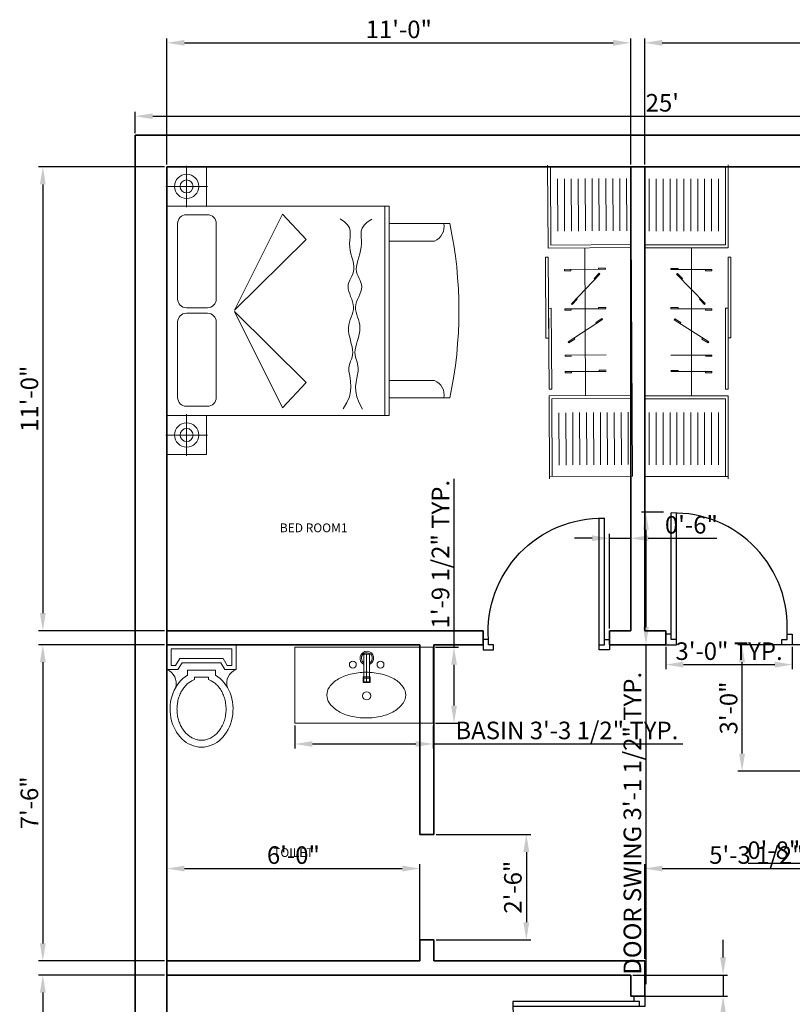
# Model space of a CAD drawing. Units: inches. Extents: x -24887 to 3061, y 1794 to 4919553.
# Tile 12 of 14: x 2721 to 2941, y 2190 to 2470. Entities that reach past the tile are written whole.
import ezdxf

# ---------------------------------------------------------------- set-up
doc = ezdxf.new("R2010")
doc.units = ezdxf.units.IN
for name, color, linetype, lineweight in [('A-ANNO-DIMS', 2, 'Continuous', 18), ('A-AREA-IDEN', 7, 'Continuous', 18), ('A-FLOR-FIXT', 9, 'Continuous', 18), ('A-FURN', 8, 'Continuous', 18), ('door', 4, 'Continuous', 25), ('wall', 7, 'Continuous', 35)]:
    doc.layers.add(name, color=color, linetype=linetype, lineweight=lineweight)
doc.styles.get("Standard").update_dxf_attribs({"font": 'arial.ttf'})
doc.dimstyles.new('ISO-25', dxfattribs={"dimtxt": 5, "dimasz": 5, "dimexe": 1.25, "dimexo": 0.625, "dimtad": 1, "dimdec": 1, "dimlunit": 3, "dimtxsty": 'Standard', "dimcen": 2.5, "dimadec": 0, "dimazin": 0, "dimtfac": 1, "dimtdec": 1, "dimtmove": 0, "dimatfit": 3, "dimfxl": 1, "dimarcsym": 0})

# ---------------------------------------------------------------- blocks, each defined once
blk = doc.blocks.new('A$C4F543DC7')
for p, q in [((0.013, 3.35, -0.169), (3.313, 3.35, -0.169)), ((0.463, 3.35, -0.169), (0.013, 3.35, -0.169)), ((0.013, 2.896, -0.169), (0.013, 3.35, -0.169)), ((0.013, 3.35, -0.169), (0.013, 2.896, -0.169)), ((0.238, 3.123, -0.439), (0.238, 3.361, -0.439)), ((0.463, 3.35, -0.169), (0.463, 0.8, -0.169)), ((2.863, 3.35, -0.169), (0.463, 3.35, -0.169)), ((0.463, 2.896, -0.169), (0.463, 3.35, -0.169)), ((2.863, 0.8, -0.169), (2.863, 3.35, -0.169)), ((2.863, 3.35, -0.169), (3.313, 3.35, -0.169)), ((2.863, 2.896, -0.169), (2.863, 3.35, -0.169)), ((3.089, 3.123, -0.439), (3.089, 3.361, -0.439)), ((3.313, 3.35, -0.169), (3.313, 2.896, -0.169)), ((3.313, 3.35, -0.169), (3.313, 2.896, -0.169)), ((1.535, 3.226, -0.169), (0.668, 3.226, -0.169)), ((2.664, 3.226, -0.169), (1.797, 3.226, -0.169)), ((0.238, 3.123, -0.439), (0, 3.123, -0.439)), ((0.238, 3.123, -0.439), (0.476, 3.123, -0.439)), ((0.238, 3.123, -0.439), (0.238, 2.885, -0.439)), ((0.568, 3.126, -0.169), (0.568, 2.884, -0.169)), ((1.635, 2.884, -0.169), (1.635, 3.126, -0.169)), ((1.697, 3.126, -0.169), (1.697, 2.884, -0.169)), ((2.764, 2.884, -0.169), (2.764, 3.126, -0.169)), ((3.089, 3.123, -0.439), (2.851, 3.123, -0.439)), ((3.089, 3.123, -0.439), (3.089, 2.885, -0.439)), ((3.089, 3.123, -0.439), (3.327, 3.123, -0.439)), ((0.463, 2.896, -0.169), (0.013, 2.896, -0.169)), ((0.013, 2.896, -0.169), (0.463, 2.896, -0.169)), ((0.463, 0.8, -0.169), (0.463, 2.896, -0.169)), ((2.863, 2.896, -0.169), (2.863, 0.8, -0.169)), ((3.313, 2.896, -0.169), (2.863, 2.896, -0.169)), ((3.313, 2.896, -0.169), (2.863, 2.896, -0.169)), ((0.668, 2.784, -0.169), (1.535, 2.784, -0.169)), ((1.797, 2.784, -0.169), (2.664, 2.784, -0.169)), ((1.653, 2.573, -0.169), (0.55, 2.025, -0.169)), ((0.841, 1.752, -0.169), (1.653, 2.573, -0.169)), ((2.481, 1.752, -0.169), (1.669, 2.573, -0.169)), ((1.669, 2.573, -0.169), (2.772, 2.025, -0.169)), ((0.55, 2.025, -0.169), (0.841, 1.752, -0.169)), ((2.772, 2.025, -0.169), (2.481, 1.752, -0.169)), ((2.683, 1.312, -0.169), (2.718, 1.364, -0.169)), ((0.537, 1.327, -0.169), (0.609, 1.284, -0.169)), ((0.609, 1.284, -0.169), (0.676, 1.257, -0.169)), ((0.676, 1.257, -0.169), (0.737, 1.243, -0.169)), ((0.737, 1.243, -0.169), (0.794, 1.239, -0.169)), ((0.846, 1.242, -0.169), (0.893, 1.249, -0.169)), ((0.893, 1.249, -0.169), (0.935, 1.256, -0.169)), ((0.935, 1.256, -0.169), (0.972, 1.261, -0.169)), ((0.972, 1.261, -0.169), (1.004, 1.262, -0.169)), ((1.004, 1.262, -0.169), (1.033, 1.258, -0.169)), ((1.033, 1.258, -0.169), (1.06, 1.251, -0.169)), ((1.06, 1.251, -0.169), (1.084, 1.242, -0.169)), ((1.084, 1.242, -0.169), (1.108, 1.234, -0.169)), ((1.285, 1.235, -0.169), (1.322, 1.244, -0.169)), ((1.322, 1.244, -0.169), (1.359, 1.253, -0.169)), ((1.359, 1.253, -0.169), (1.396, 1.261, -0.169)), ((1.396, 1.261, -0.169), (1.433, 1.266, -0.169)), ((1.433, 1.266, -0.169), (1.468, 1.268, -0.169)), ((1.468, 1.268, -0.169), (1.501, 1.264, -0.169)), ((1.501, 1.264, -0.169), (1.532, 1.257, -0.169)), ((1.532, 1.257, -0.169), (1.562, 1.247, -0.169)), ((1.562, 1.247, -0.169), (1.591, 1.237, -0.169)), ((1.826, 1.242, -0.169), (1.856, 1.253, -0.169)), ((1.856, 1.253, -0.169), (1.885, 1.263, -0.169)), ((1.885, 1.263, -0.169), (1.913, 1.27, -0.169)), ((1.913, 1.27, -0.169), (1.94, 1.272, -0.169)), ((1.94, 1.272, -0.169), (1.965, 1.269, -0.169)), ((1.965, 1.269, -0.169), (1.989, 1.262, -0.169)), ((1.989, 1.262, -0.169), (2.012, 1.251, -0.169)), ((2.012, 1.251, -0.169), (2.036, 1.239, -0.169)), ((2.317, 1.238, -0.169), (2.356, 1.246, -0.169)), ((2.356, 1.246, -0.169), (2.394, 1.253, -0.169)), ((2.394, 1.253, -0.169), (2.433, 1.255, -0.169)), ((2.433, 1.255, -0.169), (2.47, 1.253, -0.169)), ((2.47, 1.253, -0.169), (2.506, 1.249, -0.169)), ((2.506, 1.249, -0.169), (2.542, 1.246, -0.169)), ((2.542, 1.246, -0.169), (2.578, 1.248, -0.169)), ((2.578, 1.248, -0.169), (2.613, 1.257, -0.169)), ((2.613, 1.257, -0.169), (2.648, 1.277, -0.169)), ((2.648, 1.277, -0.169), (2.683, 1.312, -0.169)), ((0.533, 1.105, -0.169), (0.607, 1.146, -0.169)), ((0.607, 1.146, -0.169), (0.674, 1.171, -0.169)), ((0.674, 1.171, -0.169), (0.736, 1.183, -0.169)), ((0.736, 1.183, -0.169), (0.793, 1.185, -0.169)), ((0.793, 1.185, -0.169), (0.845, 1.18, -0.169)), ((0.794, 1.239, -0.169), (0.846, 1.242, -0.169)), ((0.845, 1.18, -0.169), (0.891, 1.172, -0.169)), ((0.891, 1.172, -0.169), (0.933, 1.163, -0.169)), ((0.933, 1.163, -0.169), (0.97, 1.156, -0.169)), ((0.97, 1.156, -0.169), (1.003, 1.155, -0.169)), ((1.003, 1.155, -0.169), (1.032, 1.158, -0.169)), ((1.032, 1.158, -0.169), (1.058, 1.164, -0.169)), ((1.058, 1.164, -0.169), (1.083, 1.172, -0.169)), ((1.083, 1.172, -0.169), (1.107, 1.18, -0.169)), ((1.107, 1.18, -0.169), (1.132, 1.187, -0.169)), ((1.108, 1.234, -0.169), (1.132, 1.226, -0.169)), ((1.132, 1.226, -0.169), (1.158, 1.22, -0.169)), ((1.132, 1.187, -0.169), (1.157, 1.192, -0.169)), ((1.157, 1.192, -0.169), (1.185, 1.193, -0.169)), ((1.158, 1.22, -0.169), (1.185, 1.218, -0.169)), ((1.185, 1.218, -0.169), (1.216, 1.22, -0.169)), ((1.185, 1.193, -0.169), (1.216, 1.19, -0.169)), ((1.216, 1.22, -0.169), (1.25, 1.226, -0.169)), ((1.216, 1.19, -0.169), (1.249, 1.183, -0.169)), ((1.249, 1.183, -0.169), (1.284, 1.173, -0.169)), ((1.25, 1.226, -0.169), (1.285, 1.235, -0.169)), ((1.284, 1.173, -0.169), (1.321, 1.163, -0.169)), ((1.321, 1.163, -0.169), (1.358, 1.152, -0.169)), ((1.358, 1.152, -0.169), (1.394, 1.143, -0.169)), ((1.394, 1.143, -0.169), (1.431, 1.137, -0.169)), ((1.431, 1.137, -0.169), (1.466, 1.135, -0.169)), ((1.466, 1.135, -0.169), (1.499, 1.137, -0.169)), ((1.499, 1.137, -0.169), (1.531, 1.143, -0.169)), ((1.531, 1.143, -0.169), (1.561, 1.152, -0.169)), ((1.561, 1.152, -0.169), (1.59, 1.162, -0.169)), ((1.59, 1.162, -0.169), (1.619, 1.172, -0.169)), ((1.591, 1.237, -0.169), (1.62, 1.226, -0.169)), ((1.619, 1.172, -0.169), (1.648, 1.18, -0.169)), ((1.62, 1.226, -0.169), (1.648, 1.217, -0.169)), ((1.648, 1.217, -0.169), (1.676, 1.211, -0.169)), ((1.648, 1.18, -0.169), (1.676, 1.185, -0.169)), ((1.676, 1.211, -0.169), (1.705, 1.209, -0.169)), ((1.676, 1.185, -0.169), (1.705, 1.186, -0.169)), ((1.705, 1.209, -0.169), (1.735, 1.212, -0.169)), ((1.705, 1.186, -0.169), (1.734, 1.182, -0.169)), ((1.734, 1.182, -0.169), (1.764, 1.173, -0.169)), ((1.735, 1.212, -0.169), (1.765, 1.22, -0.169)), ((1.764, 1.173, -0.169), (1.794, 1.162, -0.169)), ((1.765, 1.22, -0.169), (1.795, 1.23, -0.169)), ((1.794, 1.162, -0.169), (1.824, 1.149, -0.169)), ((1.795, 1.23, -0.169), (1.826, 1.242, -0.169)), ((1.824, 1.149, -0.169), (1.854, 1.137, -0.169)), ((1.854, 1.137, -0.169), (1.883, 1.126, -0.169)), ((1.987, 1.124, -0.169), (2.011, 1.134, -0.169)), ((2.011, 1.134, -0.169), (2.034, 1.145, -0.169)), ((2.034, 1.145, -0.169), (2.059, 1.157, -0.169)), ((2.036, 1.239, -0.169), (2.06, 1.227, -0.169)), ((2.059, 1.157, -0.169), (2.084, 1.167, -0.169)), ((2.06, 1.227, -0.169), (2.085, 1.216, -0.169)), ((2.084, 1.167, -0.169), (2.111, 1.174, -0.169)), ((2.085, 1.216, -0.169), (2.112, 1.208, -0.169)), ((2.111, 1.174, -0.169), (2.14, 1.177, -0.169)), ((2.112, 1.208, -0.169), (2.141, 1.204, -0.169)), ((2.14, 1.177, -0.169), (2.172, 1.175, -0.169)), ((2.141, 1.204, -0.169), (2.172, 1.205, -0.169)), ((2.172, 1.205, -0.169), (2.206, 1.21, -0.169)), ((2.172, 1.175, -0.169), (2.206, 1.169, -0.169)), ((2.206, 1.21, -0.169), (2.242, 1.218, -0.169)), ((2.206, 1.169, -0.169), (2.241, 1.16, -0.169)), ((2.241, 1.16, -0.169), (2.278, 1.149, -0.169)), ((2.242, 1.218, -0.169), (2.279, 1.228, -0.169)), ((2.278, 1.149, -0.169), (2.316, 1.138, -0.169)), ((2.279, 1.228, -0.169), (2.317, 1.238, -0.169)), ((2.316, 1.138, -0.169), (2.354, 1.128, -0.169)), ((1.883, 1.126, -0.169), (1.911, 1.119, -0.169)), ((1.911, 1.119, -0.169), (1.937, 1.115, -0.169)), ((1.937, 1.115, -0.169), (1.963, 1.118, -0.169)), ((1.963, 1.118, -0.169), (1.987, 1.124, -0.169)), ((2.354, 1.128, -0.169), (2.392, 1.121, -0.169)), ((2.392, 1.121, -0.169), (2.43, 1.117, -0.169)), ((2.43, 1.117, -0.169), (2.468, 1.118, -0.169)), ((2.468, 1.118, -0.169), (2.504, 1.121, -0.169)), ((2.504, 1.121, -0.169), (2.54, 1.123, -0.169)), ((2.54, 1.123, -0.169), (2.576, 1.12, -0.169)), ((2.576, 1.12, -0.169), (2.611, 1.109, -0.169)), ((2.611, 1.109, -0.169), (2.645, 1.088, -0.169)), ((2.645, 1.088, -0.169), (2.679, 1.052, -0.169)), ((2.679, 1.052, -0.169), (2.712, 0.999, -0.169)), ((0.463, 0.85, -0.169), (2.863, 0.85, -0.169)), ((0.463, 0.8, -0.169), (2.863, 0.8, -0.169)), ((0.663, 0.8, -0.169), (0.463, 0.8, -0.169)), ((0.663, 0.8, -0.169), (2.663, 0.8, -0.169)), ((0.663, 0.104, -0.169), (0.663, 0.8, -0.169)), ((0.663, 0.104, -0.169), (0.663, 0.8, -0.169)), ((0.863, 0.281, -0.169), (0.863, 0.8, -0.169)), ((2.463, 0.8, -0.169), (2.463, 0.281, -0.169)), ((2.863, 0.8, -0.169), (2.663, 0.8, -0.169)), ((2.663, 0.8, -0.169), (2.663, 0.104, -0.169)), ((2.663, 0.8, -0.169), (2.663, 0.104, -0.169))]:
    blk.add_line(p, q)
for centre, radius in [((0.238, 3.123, -0.439), 0.139), ((0.238, 3.123, -0.439), 0.075), ((3.089, 3.123, -0.439), 0.139), ((3.089, 3.123, -0.439), 0.075)]:
    blk.add_circle(centre, radius)
for centre, radius, start, end in [((0.668, 3.126, -0.169), 0.1, 90, 180), ((1.535, 3.126, -0.169), 0.1, 0, 90), ((1.797, 3.126, -0.169), 0.1, 90, 180), ((2.664, 3.126, -0.169), 0.1, 0, 90), ((0.668, 2.884, -0.169), 0.1, 180, 270), ((1.535, 2.884, -0.169), 0.1, 270, 0), ((1.797, 2.884, -0.169), 0.1, 180, 270), ((2.664, 2.884, -0.169), 0.1, 270, 0), ((0.699, 0.347, -0.169), 0.177, 258.2616, 338.032), ((2.627, 0.347, -0.169), 0.177, 201.968, 281.7384), ((1.663, 4.86, -0.169), 4.86, 258.1252, 281.8748), ((1.663, 4.86, -0.169), 4.86, 258.1252, 281.8748)]:
    blk.add_arc(centre, radius, start, end)
blk = doc.blocks.new('A$C34930FF8')
at = {"ltscale": 0.05}
for p, q in [((0, 2252.4), (0, 16.8)), ((600, 2252.4), (0, 2252.4)), ((185.4, 1513), (185.4, 1521.5)), ((237.7, 1513), (237.7, 1521.5)), ((436.7, 1513), (436.7, 1504.4)), ((482.5, 1513), (482.5, 1504.4)), ((227.1, 1479.2), (233.2, 1485.2)), ((263.6, 1441.7), (269.7, 1447.7)), ((398.2, 1303.6), (392.1, 1297.6)), ((185.4, 1229.1), (185.4, 1237.7)), ((237.7, 1229.1), (237.7, 1237.7)), ((434.8, 1266.1), (428.7, 1260.1)), ((436.7, 1228.2), (436.7, 1219.7)), ((482.5, 1228.2), (482.5, 1219.7)), ((209.5, 1150.1), (214.1, 1157.3)), ((253.5, 1121.8), (258.1, 1129)), ((415.3, 1017.6), (410.6, 1010.5)), ((459.3, 989.3), (454.7, 982.1)), ((482.5, 894.9), (482.5, 886.3)), ((237.7, 775.3), (237.7, 783.9)), ((436.7, 775.3), (436.7, 766.8)), ((482.5, 775.3), (482.5, 766.8)), ((600, 16.8), (0, 16.8))]:
    blk.add_line(p, q, dxfattribs=at)
for p, q in [((580, 1690.9), (580, 2252.4)), ((600, 1669.3), (600, 2269.3)), ((30, 1790.9), (30, 2169.3)), ((80, 1790.9), (80, 2169.3)), ((130, 1790.9), (130, 2169.3)), ((180, 1790.9), (180, 2169.3)), ((230, 1790.9), (230, 2169.3)), ((280, 1790.9), (280, 2169.3)), ((330, 1790.9), (330, 2169.3)), ((380, 1790.9), (380, 2169.3)), ((430, 1790.9), (430, 2169.3)), ((480, 1790.9), (480, 2169.3)), ((530, 1790.9), (530, 2169.3)), ((580, 1690.9), (0, 1690.9)), ((600, 1669.3), (0, 1669.3)), ((335.4, 1666.1), (335.4, 603.1)), ((600, 1603.3), (620, 1603.3)), ((600, 1018.7), (600, 1603.3)), ((620, 1603.3), (620, 1018.7)), ((237.7, 1521.5), (185.4, 1521.5)), ((482.5, 1513), (185.4, 1513)), ((436.7, 1504.4), (482.5, 1504.4)), ((434.8, 1266.1), (227.4, 1478.9)), ((269.7, 1447.7), (233.2, 1485.2)), ((428.7, 1260.1), (392.1, 1297.6)), ((237.7, 1237.7), (185.4, 1237.7)), ((482.5, 1228.2), (185.4, 1228.2)), ((436.7, 1219.7), (482.5, 1219.7)), ((600, 1233.4), (580, 1233.4)), ((580, 1233.4), (580, 648.7)), ((600, 648.7), (600, 1233.4)), ((459.3, 989.3), (209.5, 1150.1)), ((258.1, 1129), (214.1, 1157.3)), ((454.7, 982.1), (410.6, 1010.5)), ((620, 1018.7), (600, 1018.7)), ((482.5, 894.9), (185.4, 894.9)), ((436.7, 886.3), (482.5, 886.3)), ((237.7, 783.9), (185.4, 783.9)), ((482.5, 775.3), (185.4, 775.3)), ((436.7, 766.8), (482.5, 766.8)), ((580, 648.7), (600, 648.7)), ((600, 600), (0, 600)), ((580, 578.3), (0, 578.3)), ((580, 578.3), (580, 16.8)), ((600, 600), (600, 0)), ((30, 478.3), (30, 100)), ((80, 478.3), (80, 100)), ((130, 478.3), (130, 100)), ((180, 478.3), (180, 100)), ((230, 478.3), (230, 100)), ((280, 478.3), (280, 100)), ((330, 478.3), (330, 100)), ((380, 478.3), (380, 100)), ((430, 478.3), (430, 100)), ((480, 478.3), (480, 100)), ((530, 478.3), (530, 100))]:
    blk.add_line(p, q)
blk = doc.blocks.new('A$C7C8779AE')
for p, q in [((0, 0.7405), (0, 0.5605)), ((0.5, 0.7405), (0, 0.7405)), ((0.5, 0.5605), (0.5, 0.7405)), ((0.47, 0.7105), (0.03, 0.7105)), ((0.03, 0.7105), (0.03, 0.5905)), ((0.47, 0.5905), (0.47, 0.7105)), ((0.03, 0.5905), (0.063, 0.5905)), ((0.093, 0.6405), (0.063, 0.5905)), ((0.11, 0.6105), (0.08, 0.5605)), ((0.093, 0.6405), (0.407, 0.6405)), ((0.11, 0.6105), (0.39, 0.6105)), ((0.42, 0.5605), (0.39, 0.6105)), ((0.437, 0.5905), (0.407, 0.6405)), ((0.437, 0.5905), (0.47, 0.5905)), ((0, 0.5605), (0.08, 0.5605)), ((0.1497, 0.557), (0.1497, 0.5203)), ((0.1497, 0.557), (0.3514, 0.557)), ((0.1997, 0.507), (0.1997, 0.4879)), ((0.1997, 0.507), (0.3014, 0.507)), ((0.3014, 0.507), (0.3014, 0.4879)), ((0.3514, 0.557), (0.3514, 0.5203)), ((0.42, 0.5605), (0.5, 0.5605))]:
    blk.add_line(p, q)
for centre, start, end in [((-0.0386, 0.4613), 344.64203, 68.73386), ((0.5386, 0.4613), 111.26614, 195.35797)]:
    blk.add_arc(centre, 0.1064, start, end)
blk.add_ellipse((0.2506, 0.2744), major_axis=(0, 0.2744), ratio=0.828948, start_param=0.459479, end_param=5.823706)
blk.add_open_spline([(0.1997, 0.4879), (0.1697, 0.474), (0.1642, 0.4702), (0.1512, 0.4602), (0.1438, 0.4535), (0.1298, 0.4388), (0.1233, 0.4306), (0.1111, 0.4131), (0.1055, 0.4037), (0.0956, 0.3838), (0.0912, 0.3733), (0.0838, 0.3516), (0.0808, 0.3403), (0.0762, 0.3172), (0.0746, 0.3055), (0.073, 0.2817), (0.0729, 0.2698), (0.0743, 0.246), (0.0758, 0.2342), (0.0801, 0.2111), (0.0831, 0.1998), (0.0903, 0.1779), (0.0945, 0.1673), (0.1043, 0.1473), (0.1098, 0.1378), (0.1218, 0.12), (0.1283, 0.1118), (0.1421, 0.0968), (0.1494, 0.09), (0.1646, 0.078), (0.1725, 0.0728), (0.1887, 0.064), (0.1969, 0.0603), (0.2137, 0.0547), (0.2222, 0.0527), (0.2392, 0.0502), (0.2478, 0.0498), (0.2664, 0.0505), (0.2764, 0.052), (0.2963, 0.0573), (0.3061, 0.061), (0.3253, 0.0707), (0.3346, 0.0766), (0.3525, 0.0906), (0.3611, 0.0987), (0.3771, 0.1169), (0.3845, 0.127), (0.3978, 0.1488), (0.4037, 0.1605), (0.4137, 0.1853), (0.4178, 0.1983), (0.424, 0.2251), (0.4261, 0.2389), (0.4282, 0.2668), (0.4283, 0.2809), (0.4262, 0.3088), (0.4241, 0.3226), (0.418, 0.3495), (0.414, 0.3625), (0.404, 0.3873), (0.3982, 0.3991), (0.385, 0.421), (0.3776, 0.4311), (0.3617, 0.4494), (0.3531, 0.4575), (0.3382, 0.4693), (0.3321, 0.4736), (0.3014, 0.4879)], degree=3, knots=[0.459479, 0.459479, 0.459479, 0.459479, 0.567422, 0.567422, 0.720865, 0.720865, 0.874307, 0.874307, 1.02775, 1.02775, 1.181192, 1.181192, 1.334635, 1.334635, 1.488077, 1.488077, 1.64152, 1.64152, 1.794963, 1.794963, 1.948405, 1.948405, 2.101848, 2.101848, 2.25529, 2.25529, 2.408733, 2.408733, 2.562175, 2.562175, 2.715618, 2.715618, 2.86906, 2.86906, 3.022503, 3.022503, 3.175946, 3.175946, 3.356457, 3.356457, 3.536968, 3.536968, 3.717479, 3.717479, 3.89799, 3.89799, 4.078501, 4.078501, 4.259012, 4.259012, 4.439523, 4.439523, 4.620035, 4.620035, 4.800546, 4.800546, 4.981057, 4.981057, 5.161568, 5.161568, 5.342079, 5.342079, 5.52259, 5.52259, 5.703101, 5.703101, 5.823706, 5.823706, 5.823706, 5.823706])
blk = doc.blocks.new('A$C50A015BB')
for p, q in [((0, 0.55), (1, 0.55)), ((0, 0.55), (0, 0)), ((0.4985, 0.5), (0.5385, 0.5)), ((0.4985, 0.5), (0.4985, 0.3)), ((0.5185, 0.5), (0.5185, 0.3)), ((0.5385, 0.5), (0.5385, 0.3)), ((1, 0.55), (1, 0)), ((0.4935, 0.335), (0.4935, 0.295)), ((0.4935, 0.335), (0.5435, 0.335)), ((0.4935, 0.295), (0.5435, 0.295)), ((0.4985, 0.325), (0.5385, 0.325)), ((0.4985, 0.3), (0.5385, 0.3)), ((0.5435, 0.335), (0.5435, 0.295)), ((0, 0), (1, 0)), ((0, 0), (1, 0))]:
    blk.add_line(p, q)
for centre, radius in [((0.4185, 0.424), 0.025), ((0.6185, 0.424), 0.025), ((0.5185, 0.1981), 0.0298)]:
    blk.add_circle(centre, radius)
for centre, radius, start, end in [((0.5201, 0.4703), 0.0497, 291.74253, 244.23308), ((0.5201, 0.4703), 0.0397, 297.63203, 237.02558), ((0.5157, -0.1225), 0.4906, 90, 103.48533), ((0.5157, -0.1225), 0.4906, 76.51467, 90), ((0.4185, 0.1397), 0.2081, 120.06859, 144.41781), ((0.4772, 0.0383), 0.3252, 103.48533, 120.06859), ((0.5543, 0.0383), 0.3252, 59.93141, 76.51467), ((0.613, 0.1397), 0.2081, 35.58219, 59.93141), ((0.3299, 0.2031), 0.0991, 144.41781, 180), ((0.7016, 0.2031), 0.0991, 0, 35.58219), ((0.3299, 0.2031), 0.0991, 180, 215.58219), ((0.4185, 0.2665), 0.2081, 215.58219, 239.93141), ((0.613, 0.2665), 0.2081, 300.06859, 324.41781), ((0.7016, 0.2031), 0.0991, 324.41781, 0), ((0.4772, 0.3679), 0.3252, 239.93141, 256.51467), ((0.5543, 0.3679), 0.3252, 283.48533, 300.06859), ((0.5157, 0.5288), 0.4906, 256.51467, 270), ((0.5157, 0.5288), 0.4906, 270, 283.48533)]:
    blk.add_arc(centre, radius, start, end)
blk = doc.blocks.new('*D32')
at = {"layer": 'A-ANNO-DIMS', "color": 0, "lineweight": -2, "transparency": 16777216}
for p, q in [((2753.93, 2437.57), (2753.93, 2443.6)), ((3053.93, 2437.57), (3053.93, 2443.6)), ((2758.93, 2442.35), (3048.93, 2442.35))]:
    blk.add_line(p, q, dxfattribs=at)
at = {"layer": 'A-ANNO-DIMS', "color": 0, "transparency": 16777216}
for points in [[(2758.93, 2443.19), (2758.93, 2441.52), (2753.93, 2442.35)], [(3048.93, 2443.19), (3048.93, 2441.52), (3053.93, 2442.35)]]:
    blk.add_solid(points, dxfattribs=at)
at = {"layer": 'Defpoints', "color": 0, "transparency": 16777216}
for p in [(3053.93, 2442.35), (2753.93, 2436.94), (3053.93, 2436.94)]:
    blk.add_point(p, dxfattribs=at)
at = {"layer": 'A-ANNO-DIMS', "color": 0, "transparency": 16777216, "insert": (2903.93, 2445.53), "char_height": 5, "attachment_point": 5}
blk.add_mtext("25'", dxfattribs=at)
blk = doc.blocks.new('DOOR-SINGLE-36IN')
for p, q in [((34.5, 36), (37.5, 36)), ((34.5, 34.5), (34.5, 36)), ((36, 34.5), (34.5, 34.5)), ((36, 33), (36, 34.5)), ((37.5, 36), (37.5, 33)), ((37.5, 33), (36, 33)), ((36, 3), (0, 3)), ((37.5, 3), (36, 3)), ((36, 3), (36, 1.5)), ((37.5, 0), (37.5, 3)), ((36, 1.5), (0, 1.5)), ((36, 1.5), (34.5, 1.5)), ((34.5, 1.5), (34.5, 0)), ((34.5, 0), (37.5, 0))]:
    blk.add_line(p, q)
blk.add_arc((32.32, 2.25), 32.32, 86.1244, 181.3295)
blk = doc.blocks.new('*D38')
at = {"layer": 'A-ANNO-DIMS', "color": 0, "lineweight": -2, "transparency": 16777216}
for p, q in [((2904.3, 2329.65), (2898.02, 2329.65)), ((2899.27, 2324.65), (2899.27, 2296.94)), ((2904.3, 2291.94), (2898.02, 2291.94)), ((2899.27, 2291.94), (2899.27, 2195.31))]:
    blk.add_line(p, q, dxfattribs=at)
at = {"layer": 'A-ANNO-DIMS', "color": 0, "transparency": 16777216}
for points in [[(2898.44, 2324.65), (2900.1, 2324.65), (2899.27, 2329.65)], [(2898.44, 2296.94), (2900.1, 2296.94), (2899.27, 2291.94)]]:
    blk.add_solid(points, dxfattribs=at)
at = {"layer": 'Defpoints', "color": 0, "transparency": 16777216}
for p in [(2904.93, 2329.65), (2899.27, 2291.94), (2904.93, 2291.94)]:
    blk.add_point(p, dxfattribs=at)
at = {"layer": 'A-ANNO-DIMS', "color": 0, "transparency": 16777216, "insert": (2896.06, 2241.12), "char_height": 5, "attachment_point": 5, "rotation": 90}
blk.add_mtext('DOOR SWING 3\'-1 1/2" TYP.', dxfattribs=at)
blk = doc.blocks.new('*D39')
at = {"layer": 'A-ANNO-DIMS', "color": 0, "lineweight": -2, "transparency": 16777216}
for p, q in [((2904.93, 2291.32), (2904.93, 2285.03)), ((2940.93, 2291.32), (2940.93, 2285.03)), ((2909.93, 2286.28), (2935.93, 2286.28))]:
    blk.add_line(p, q, dxfattribs=at)
at = {"layer": 'A-ANNO-DIMS', "color": 0, "transparency": 16777216}
for points in [[(2909.93, 2287.12), (2909.93, 2285.45), (2904.93, 2286.28)], [(2935.93, 2287.12), (2935.93, 2285.45), (2940.93, 2286.28)]]:
    blk.add_solid(points, dxfattribs=at)
at = {"layer": 'Defpoints', "color": 0, "transparency": 16777216}
for p in [(2904.93, 2291.94), (2940.93, 2291.94), (2940.93, 2286.28)]:
    blk.add_point(p, dxfattribs=at)
at = {"layer": 'A-ANNO-DIMS', "color": 0, "transparency": 16777216, "insert": (2922.93, 2289.46), "char_height": 5, "attachment_point": 5}
blk.add_mtext('3\'-0" TYP.', dxfattribs=at)
blk = doc.blocks.new('*D46')
at = {"layer": 'A-ANNO-DIMS', "color": 0, "lineweight": -2, "transparency": 16777216}
for p, q in [((2799.37, 2268.97), (2799.37, 2262.44)), ((2838.74, 2268.97), (2838.74, 2262.44)), ((2804.37, 2263.69), (2833.74, 2263.69)), ((2838.74, 2263.69), (2909.8, 2263.69))]:
    blk.add_line(p, q, dxfattribs=at)
at = {"layer": 'A-ANNO-DIMS', "color": 0, "transparency": 16777216}
for points in [[(2804.37, 2264.52), (2804.37, 2262.86), (2799.37, 2263.69)], [(2833.74, 2264.52), (2833.74, 2262.86), (2838.74, 2263.69)]]:
    blk.add_solid(points, dxfattribs=at)
at = {"layer": 'Defpoints', "color": 0, "transparency": 16777216}
for p in [(2799.37, 2269.6), (2838.74, 2269.6), (2838.74, 2263.69)]:
    blk.add_point(p, dxfattribs=at)
at = {"layer": 'A-ANNO-DIMS', "color": 0, "transparency": 16777216, "insert": (2876.77, 2266.9), "char_height": 5, "attachment_point": 5}
blk.add_mtext('BASIN 3\'-3 1/2" TYP.', dxfattribs=at)
blk = doc.blocks.new('*D47')
at = {"layer": 'A-ANNO-DIMS', "color": 0, "lineweight": -2, "transparency": 16777216}
for p, q in [((2844.65, 2291.25), (2844.65, 2339.16)), ((2839.37, 2291.25), (2845.9, 2291.25)), ((2844.65, 2274.6), (2844.65, 2286.25)), ((2839.37, 2269.6), (2845.9, 2269.6))]:
    blk.add_line(p, q, dxfattribs=at)
at = {"layer": 'A-ANNO-DIMS', "color": 0, "transparency": 16777216}
for points in [[(2843.82, 2286.25), (2845.48, 2286.25), (2844.65, 2291.25)], [(2843.82, 2274.6), (2845.48, 2274.6), (2844.65, 2269.6)]]:
    blk.add_solid(points, dxfattribs=at)
at = {"layer": 'Defpoints', "color": 0, "transparency": 16777216}
for p in [(2838.74, 2291.25), (2844.65, 2291.25), (2838.74, 2269.6)]:
    blk.add_point(p, dxfattribs=at)
at = {"layer": 'A-ANNO-DIMS', "color": 0, "transparency": 16777216, "insert": (2841.44, 2317.7), "char_height": 5, "attachment_point": 5, "rotation": 90}
blk.add_mtext('1\'-9 1/2" TYP.', dxfattribs=at)
blk = doc.blocks.new('*D99')
at = {"layer": 'A-ANNO-DIMS', "color": 0, "lineweight": -2, "transparency": 16777216}
for p, q in [((2762.93, 2428.57), (2762.93, 2464.49)), ((2767.93, 2463.24), (2889.93, 2463.24)), ((2894.93, 2428.57), (2894.93, 2464.49))]:
    blk.add_line(p, q, dxfattribs=at)
at = {"layer": 'A-ANNO-DIMS', "color": 0, "transparency": 16777216}
for points in [[(2767.93, 2464.07), (2767.93, 2462.41), (2762.93, 2463.24)], [(2889.93, 2464.07), (2889.93, 2462.41), (2894.93, 2463.24)]]:
    blk.add_solid(points, dxfattribs=at)
at = {"layer": 'Defpoints', "color": 0, "transparency": 16777216}
for p in [(2894.93, 2463.24), (2762.93, 2427.94), (2894.93, 2427.94)]:
    blk.add_point(p, dxfattribs=at)
at = {"layer": 'A-ANNO-DIMS', "color": 0, "transparency": 16777216, "insert": (2828.93, 2466.42), "char_height": 5, "attachment_point": 5}
blk.add_mtext('11\'-0"', dxfattribs=at)
blk = doc.blocks.new('*D100')
at = {"layer": 'A-ANNO-DIMS', "color": 0, "lineweight": -2, "transparency": 16777216}
for p, q in [((2898.93, 2428.57), (2898.93, 2464.49)), ((2903.93, 2463.24), (3039.93, 2463.24)), ((3044.93, 2428.57), (3044.93, 2464.49))]:
    blk.add_line(p, q, dxfattribs=at)
at = {"layer": 'A-ANNO-DIMS', "color": 0, "transparency": 16777216}
for points in [[(2903.93, 2464.07), (2903.93, 2462.41), (2898.93, 2463.24)], [(3039.93, 2464.07), (3039.93, 2462.41), (3044.93, 2463.24)]]:
    blk.add_solid(points, dxfattribs=at)
at = {"layer": 'Defpoints', "color": 0, "transparency": 16777216}
for p in [(3044.93, 2463.24), (2898.93, 2427.94), (3044.93, 2427.94)]:
    blk.add_point(p, dxfattribs=at)
at = {"layer": 'A-ANNO-DIMS', "color": 0, "transparency": 16777216, "insert": (2971.93, 2466.38), "char_height": 5, "attachment_point": 5}
blk.add_mtext('12\'-2"', dxfattribs=at)
blk = doc.blocks.new('*D101')
at = {"layer": 'A-ANNO-DIMS', "color": 0, "lineweight": -2, "transparency": 16777216}
for p, q in [((2762.93, 2202.57), (2762.93, 2229.49)), ((2767.93, 2228.24), (2829.93, 2228.24)), ((2834.93, 2202.57), (2834.93, 2229.49))]:
    blk.add_line(p, q, dxfattribs=at)
at = {"layer": 'A-ANNO-DIMS', "color": 0, "transparency": 16777216}
for points in [[(2767.93, 2229.07), (2767.93, 2227.41), (2762.93, 2228.24)], [(2829.93, 2229.07), (2829.93, 2227.41), (2834.93, 2228.24)]]:
    blk.add_solid(points, dxfattribs=at)
at = {"layer": 'Defpoints', "color": 0, "transparency": 16777216}
for p in [(2834.93, 2228.24), (2762.93, 2201.94), (2834.93, 2201.94)]:
    blk.add_point(p, dxfattribs=at)
at = {"layer": 'A-ANNO-DIMS', "color": 0, "transparency": 16777216, "insert": (2798.93, 2231.42), "char_height": 5, "attachment_point": 5}
blk.add_mtext('6\'-0"', dxfattribs=at)
blk = doc.blocks.new('*D102')
at = {"layer": 'A-ANNO-DIMS', "color": 0, "lineweight": -2, "transparency": 16777216}
for p, q in [((2762.3, 2427.94), (2726.38, 2427.94)), ((2727.63, 2422.94), (2727.63, 2300.94)), ((2762.3, 2295.94), (2726.38, 2295.94))]:
    blk.add_line(p, q, dxfattribs=at)
at = {"layer": 'A-ANNO-DIMS', "color": 0, "transparency": 16777216}
for points in [[(2726.79, 2422.94), (2728.46, 2422.94), (2727.63, 2427.94)], [(2726.79, 2300.94), (2728.46, 2300.94), (2727.63, 2295.94)]]:
    blk.add_solid(points, dxfattribs=at)
at = {"layer": 'Defpoints', "color": 0, "transparency": 16777216}
for p in [(2762.93, 2427.94), (2727.63, 2295.94), (2762.93, 2295.94)]:
    blk.add_point(p, dxfattribs=at)
at = {"layer": 'A-ANNO-DIMS', "color": 0, "transparency": 16777216, "insert": (2724.45, 2361.94), "char_height": 5, "attachment_point": 5, "rotation": 90}
blk.add_mtext('11\'-0"', dxfattribs=at)
blk = doc.blocks.new('*D103')
at = {"layer": 'A-ANNO-DIMS', "color": 0, "lineweight": -2, "transparency": 16777216}
for p, q in [((2762.3, 2291.94), (2726.38, 2291.94)), ((2727.63, 2286.94), (2727.63, 2206.94)), ((2762.3, 2201.94), (2726.38, 2201.94))]:
    blk.add_line(p, q, dxfattribs=at)
at = {"layer": 'A-ANNO-DIMS', "color": 0, "transparency": 16777216}
for points in [[(2726.79, 2286.94), (2728.46, 2286.94), (2727.63, 2291.94)], [(2726.79, 2206.94), (2728.46, 2206.94), (2727.63, 2201.94)]]:
    blk.add_solid(points, dxfattribs=at)
at = {"layer": 'Defpoints', "color": 0, "transparency": 16777216}
for p in [(2762.93, 2291.94), (2727.63, 2201.94), (2762.93, 2201.94)]:
    blk.add_point(p, dxfattribs=at)
at = {"layer": 'A-ANNO-DIMS', "color": 0, "transparency": 16777216, "insert": (2724.45, 2246.94), "char_height": 5, "attachment_point": 5, "rotation": 90}
blk.add_mtext('7\'-6"', dxfattribs=at)
blk = doc.blocks.new('*D104')
at = {"layer": 'A-ANNO-DIMS', "color": 0, "lineweight": -2, "transparency": 16777216}
for p, q in [((2762.3, 2197.94), (2726.38, 2197.94)), ((2727.63, 2192.94), (2727.63, 2130.94)), ((2762.3, 2125.94), (2726.38, 2125.94))]:
    blk.add_line(p, q, dxfattribs=at)
at = {"layer": 'A-ANNO-DIMS', "color": 0, "transparency": 16777216}
for points in [[(2726.79, 2192.94), (2728.46, 2192.94), (2727.63, 2197.94)], [(2726.79, 2130.94), (2728.46, 2130.94), (2727.63, 2125.94)]]:
    blk.add_solid(points, dxfattribs=at)
at = {"layer": 'Defpoints', "color": 0, "transparency": 16777216}
for p in [(2762.93, 2197.94), (2727.63, 2125.94), (2762.93, 2125.94)]:
    blk.add_point(p, dxfattribs=at)
at = {"layer": 'A-ANNO-DIMS', "color": 0, "transparency": 16777216, "insert": (2724.45, 2161.94), "char_height": 5, "attachment_point": 5, "rotation": 90}
blk.add_mtext('6\'-0"', dxfattribs=at)
blk = doc.blocks.new('*D108')
at = {"layer": 'A-ANNO-DIMS', "color": 0, "lineweight": -2, "transparency": 16777216}
for p, q in [((2839.55, 2237.94), (2866.48, 2237.94)), ((2865.23, 2232.94), (2865.23, 2212.94)), ((2839.55, 2207.94), (2866.48, 2207.94))]:
    blk.add_line(p, q, dxfattribs=at)
at = {"layer": 'A-ANNO-DIMS', "color": 0, "transparency": 16777216}
for points in [[(2864.39, 2232.94), (2866.06, 2232.94), (2865.23, 2237.94)], [(2864.39, 2212.94), (2866.06, 2212.94), (2865.23, 2207.94)]]:
    blk.add_solid(points, dxfattribs=at)
at = {"layer": 'Defpoints', "color": 0, "transparency": 16777216}
for p in [(2838.93, 2237.94), (2838.93, 2207.94), (2865.23, 2207.94)]:
    blk.add_point(p, dxfattribs=at)
at = {"layer": 'A-ANNO-DIMS', "color": 0, "transparency": 16777216, "insert": (2862.05, 2222.94), "char_height": 5, "attachment_point": 5, "rotation": 90}
blk.add_mtext('2\'-6"', dxfattribs=at)
blk = doc.blocks.new('*D110')
at = {"layer": 'A-ANNO-DIMS', "color": 0, "lineweight": -2, "transparency": 16777216}
for p, q in [((2952.93, 2255.32), (2952.93, 2228.39)), ((2960.93, 2255.32), (2960.93, 2228.39)), ((2947.93, 2229.64), (2928.38, 2229.64)), ((2960.93, 2229.64), (2952.93, 2229.64)), ((2965.93, 2229.64), (2970.93, 2229.64))]:
    blk.add_line(p, q, dxfattribs=at)
at = {"layer": 'A-ANNO-DIMS', "color": 0, "transparency": 16777216}
for points in [[(2947.93, 2230.47), (2947.93, 2228.81), (2952.93, 2229.64)], [(2965.93, 2230.47), (2965.93, 2228.81), (2960.93, 2229.64)]]:
    blk.add_solid(points, dxfattribs=at)
at = {"layer": 'Defpoints', "color": 0, "transparency": 16777216}
for p in [(2952.93, 2255.94), (2960.93, 2255.94), (2952.93, 2229.64)]:
    blk.add_point(p, dxfattribs=at)
at = {"layer": 'A-ANNO-DIMS', "color": 0, "transparency": 16777216, "insert": (2935.66, 2232.82), "char_height": 5, "attachment_point": 5}
blk.add_mtext('0\'-8"', dxfattribs=at)
blk = doc.blocks.new('*D111')
at = {"layer": 'A-ANNO-DIMS', "color": 0, "lineweight": -2, "transparency": 16777216}
for p, q in [((2952.3, 2291.94), (2925.38, 2291.94)), ((2926.63, 2260.94), (2926.63, 2286.94)), ((2952.3, 2255.94), (2925.38, 2255.94))]:
    blk.add_line(p, q, dxfattribs=at)
at = {"layer": 'A-ANNO-DIMS', "color": 0, "transparency": 16777216}
for points in [[(2925.79, 2286.94), (2927.46, 2286.94), (2926.63, 2291.94)], [(2925.79, 2260.94), (2927.46, 2260.94), (2926.63, 2255.94)]]:
    blk.add_solid(points, dxfattribs=at)
at = {"layer": 'Defpoints', "color": 0, "transparency": 16777216}
for p in [(2926.63, 2291.94), (2952.93, 2291.94), (2952.93, 2255.94)]:
    blk.add_point(p, dxfattribs=at)
at = {"layer": 'A-ANNO-DIMS', "color": 0, "transparency": 16777216, "insert": (2923.45, 2273.94), "char_height": 5, "attachment_point": 5, "rotation": 90}
blk.add_mtext('3\'-0"', dxfattribs=at)
blk = doc.blocks.new('*D112')
at = {"layer": 'A-ANNO-DIMS', "color": 0, "lineweight": -2, "transparency": 16777216}
for p, q in [((2898.93, 2202.57), (2898.93, 2229.49)), ((2903.93, 2228.24), (2957.46, 2228.24)), ((2962.46, 2202.57), (2962.46, 2229.49))]:
    blk.add_line(p, q, dxfattribs=at)
at = {"layer": 'A-ANNO-DIMS', "color": 0, "transparency": 16777216}
for points in [[(2903.93, 2229.07), (2903.93, 2227.41), (2898.93, 2228.24)], [(2957.46, 2229.07), (2957.46, 2227.41), (2962.46, 2228.24)]]:
    blk.add_solid(points, dxfattribs=at)
at = {"layer": 'Defpoints', "color": 0, "transparency": 16777216}
for p in [(2962.46, 2228.24), (2898.93, 2201.94), (2962.46, 2201.94)]:
    blk.add_point(p, dxfattribs=at)
at = {"layer": 'A-ANNO-DIMS', "color": 0, "transparency": 16777216, "insert": (2930.69, 2231.45), "char_height": 5, "attachment_point": 5}
blk.add_mtext('5\'-3 1/2"', dxfattribs=at)
blk = doc.blocks.new('*D113')
at = {"layer": 'A-ANNO-DIMS', "color": 0, "lineweight": -2, "transparency": 16777216}
for p, q in [((2888.93, 2296.57), (2888.93, 2323.49)), ((2894.93, 2296.57), (2894.93, 2323.49)), ((2883.93, 2322.24), (2878.93, 2322.24)), ((2888.93, 2322.24), (2894.93, 2322.24)), ((2899.93, 2322.24), (2919.47, 2322.24))]:
    blk.add_line(p, q, dxfattribs=at)
at = {"layer": 'A-ANNO-DIMS', "color": 0, "transparency": 16777216}
for points in [[(2883.93, 2323.07), (2883.93, 2321.41), (2888.93, 2322.24)], [(2899.93, 2323.07), (2899.93, 2321.41), (2894.93, 2322.24)]]:
    blk.add_solid(points, dxfattribs=at)
at = {"layer": 'Defpoints', "color": 0, "transparency": 16777216}
for p in [(2894.93, 2322.24), (2888.93, 2295.94), (2894.93, 2295.94)]:
    blk.add_point(p, dxfattribs=at)
at = {"layer": 'A-ANNO-DIMS', "color": 0, "transparency": 16777216, "insert": (2912.2, 2325.42), "char_height": 5, "attachment_point": 5}
blk.add_mtext('0\'-6"', dxfattribs=at)
blk = doc.blocks.new('*D114')
at = {"layer": 'A-ANNO-DIMS', "color": 0, "lineweight": -2, "transparency": 16777216}
for p, q in [((2921.23, 2202.94), (2921.23, 2207.94)), ((2895.55, 2197.94), (2922.48, 2197.94)), ((2921.23, 2197.94), (2921.23, 2191.94)), ((2895.55, 2191.94), (2922.48, 2191.94)), ((2921.23, 2186.94), (2921.23, 2167.4))]:
    blk.add_line(p, q, dxfattribs=at)
at = {"layer": 'A-ANNO-DIMS', "color": 0, "transparency": 16777216}
for points in [[(2920.39, 2202.94), (2922.06, 2202.94), (2921.23, 2197.94)], [(2920.39, 2186.94), (2922.06, 2186.94), (2921.23, 2191.94)]]:
    blk.add_solid(points, dxfattribs=at)
at = {"layer": 'Defpoints', "color": 0, "transparency": 16777216}
for p in [(2894.93, 2197.94), (2894.93, 2191.94), (2921.23, 2191.94)]:
    blk.add_point(p, dxfattribs=at)
at = {"layer": 'A-ANNO-DIMS', "color": 0, "transparency": 16777216, "insert": (2918.05, 2174.67), "char_height": 5, "attachment_point": 5, "rotation": 90}
blk.add_mtext('0\'-6"', dxfattribs=at)

msp = doc.modelspace()

# ---------------------------------------------------------------- linework, layer by layer
at = {"layer": 'wall'}
for p, q in [((3053.93, 2436.94), (2753.93, 2436.94)), ((2753.93, 2436.94), (2753.93, 1956.94)), ((3044.93, 2427.94), (2762.93, 2427.94)), ((2762.93, 2427.94), (2762.93, 1965.94)), ((2894.93, 2427.94), (2894.93, 2295.94)), ((2898.93, 2427.94), (2898.93, 2295.94)), ((2852.93, 2295.94), (2762.93, 2295.94)), ((2852.93, 2295.94), (2852.93, 2291.94)), ((2894.93, 2295.94), (2888.93, 2295.94)), ((2888.93, 2295.94), (2888.93, 2291.94)), ((2904.93, 2295.94), (2898.93, 2295.94)), ((2904.93, 2295.94), (2904.93, 2291.94)), ((2834.93, 2291.94), (2762.93, 2291.94)), ((2834.93, 2291.94), (2834.93, 2237.94)), ((2838.93, 2291.94), (2838.93, 2237.94)), ((2852.93, 2291.94), (2838.93, 2291.94)), ((2904.93, 2291.94), (2888.93, 2291.94)), ((2834.93, 2237.94), (2838.93, 2237.94)), ((2834.93, 2207.94), (2838.93, 2207.94)), ((2834.93, 2207.94), (2834.93, 2201.94)), ((2838.93, 2207.94), (2838.93, 2201.94)), ((2834.93, 2201.94), (2762.93, 2201.94)), ((2898.93, 2201.94), (2838.93, 2201.94)), ((2898.93, 2201.94), (2898.93, 2191.94)), ((2894.93, 2197.94), (2762.93, 2197.94)), ((2894.93, 2197.94), (2894.93, 2191.94)), ((2894.93, 2191.94), (2898.93, 2191.94))]:
    msp.add_line(p, q, dxfattribs=at)

# ---------------------------------------------------------------- block references
at = {"layer": 'A-FLOR-FIXT', "xscale": 39.37007874015748, "yscale": 39.37007874015748, "zscale": 39.37007874015748}
for name, p in [('A$C7C8779AE', (2762.93, 2262.79)), ('A$C50A015BB', (2799.37, 2269.6))]:
    msp.add_blockref(name, p, dxfattribs=at)
at = {"layer": 'A-FURN'}
for name, p, xscale, yscale, zscale, rotation in [('A$C4F543DC7', (2846.05, 2345.72, 4.19), 24.81469674658305, 24.81469674658305, 24.81469674658305, 90), ('A$C34930FF8', (2895.46, 2339.26), -0.0393700787401575, 0.0393700787401575, 0.0393700787401575, 0.3450343303282022)]:
    msp.add_blockref(name, p, dxfattribs=dict(at, xscale=xscale, yscale=yscale, zscale=zscale, rotation=rotation))
at = {"layer": 'A-FURN', "xscale": 0.0393700787401575, "yscale": 0.0393700787401575, "zscale": 0.0393700787401575}
msp.add_blockref('A$C34930FF8', (2899.05, 2339.16), dxfattribs=at)
at = {"layer": 'door', "rotation": 269.9999999999987}
msp.add_blockref('DOOR-SINGLE-36IN', (2904.93, 2329.44), dxfattribs=at)
at = {"layer": 'door', "extrusion": (0, 0, -1), "zscale": -1}
for p, rotation in [((-2888.93, 2327.94), 270.0000000000034), ((-2861.43, 2191.94), 180)]:
    msp.add_blockref('DOOR-SINGLE-36IN', p, dxfattribs=dict(at, rotation=rotation))

# ---------------------------------------------------------------- texts
at = {"layer": 'A-AREA-IDEN', "char_height": 2.5, "attachment_point": 1}
for s, insert in [('BED ROOM1', (2795.08, 2326.46)), ('TOILET', (2793.18, 2234.03))]:
    msp.add_mtext_dynamic_manual_height_columns(s, width=34.2323, gutter_width=12.5, heights=[0], dxfattribs=dict(at, insert=insert))

# ---------------------------------------------------------------- dimensions: what is measured, and where the dimension line sits
at = {"layer": 'A-ANNO-DIMS'}
for base, p1, p2, override, picture, middle in [((2894.93, 2463.24), (2762.93, 2427.94), (2894.93, 2427.94), {"dimdec": 1, "dimlfac": 1, "dimrnd": 0, "dimzin": 1, "dimdsep": 46, "dimlunit": 4, "dimfrac": 2}, '*D99', (2828.93, 2466.42)), ((3044.93, 2463.24), (2898.93, 2427.94), (3044.93, 2427.94), {"dimdec": 1, "dimlfac": 1, "dimrnd": 0, "dimzin": 1, "dimdsep": 46, "dimlunit": 4, "dimfrac": 2}, '*D100', (2971.93, 2466.38)), ((3053.93, 2442.35), (2753.93, 2436.94), (3053.93, 2436.94), {"dimclrd": 0, "dimclre": 0, "dimclrt": 0}, '*D32', (2903.93, 2445.53)), ((2894.93, 2322.24), (2888.93, 2295.94), (2894.93, 2295.94), {"dimdec": 1, "dimlfac": 1, "dimrnd": 0, "dimzin": 1, "dimdsep": 46, "dimlunit": 4, "dimfrac": 2}, '*D113', (2912.2, 2325.42)), ((2962.46, 2228.24), (2898.93, 2201.94), (2962.46, 2201.94), {"dimdec": 1, "dimlfac": 1, "dimrnd": 0, "dimzin": 1, "dimdsep": 46, "dimlunit": 4, "dimfrac": 2}, '*D112', (2930.69, 2231.45)), ((2834.93, 2228.24), (2762.93, 2201.94), (2834.93, 2201.94), {"dimdec": 1, "dimlfac": 1, "dimrnd": 0, "dimzin": 1, "dimdsep": 46, "dimlunit": 4, "dimfrac": 2}, '*D101', (2798.93, 2231.42))]:
    dim = msp.add_linear_dim(base=base, p1=p1, p2=p2, dimstyle='ISO-25', override=override, dxfattribs=at)
    dim.commit()
    dim.dimension.update_dxf_attribs({"geometry": picture, "text_midpoint": middle})
for base, p1, p2, angle, picture, middle in [((2727.63, 2295.94), (2762.93, 2427.94), (2762.93, 2295.94), 90, '*D102', (2724.45, 2361.94)), ((2727.63, 2201.94), (2762.93, 2291.94), (2762.93, 2201.94), 90, '*D103', (2724.45, 2246.94)), ((2926.63, 2291.94), (2952.93, 2255.94), (2952.93, 2291.94), 90, '*D111', (2923.45, 2273.94)), ((2952.93, 2229.64), (2960.93, 2255.94), (2952.93, 2255.94), 180, '*D110', (2935.66, 2232.82)), ((2865.23, 2207.94), (2838.93, 2237.94), (2838.93, 2207.94), 270, '*D108', (2862.05, 2222.94)), ((2921.23, 2191.94), (2894.93, 2197.94), (2894.93, 2191.94), 270, '*D114', (2918.05, 2174.67)), ((2727.63, 2125.94), (2762.93, 2197.94), (2762.93, 2125.94), 90, '*D104', (2724.45, 2161.94))]:
    dim = msp.add_linear_dim(base=base, p1=p1, p2=p2, angle=angle, dimstyle='ISO-25', override={"dimdec": 1, "dimlfac": 1, "dimrnd": 0, "dimzin": 1, "dimdsep": 46, "dimlunit": 4, "dimfrac": 2}, dxfattribs=at)
    dim.commit()
    dim.dimension.update_dxf_attribs({"geometry": picture, "text_midpoint": middle})
for base, p1, p2, angle, text, picture, middle in [((2844.6493, 2291.2486), (2838.7438, 2269.595), (2838.7438, 2291.2486), 90, '<> TYP.', '*D47', (2841.4391, 2317.7023)), ((2899.27, 2291.94), (2904.93, 2329.65), (2904.93, 2291.94), 270, 'DOOR SWING <> TYP.', '*D38', (2896.06, 2241.12))]:
    dim = msp.add_linear_dim(base=base, p1=p1, p2=p2, angle=angle, text=text, dimstyle='ISO-25', override={"dimdec": 1, "dimlfac": 1, "dimrnd": 0, "dimzin": 1, "dimdsep": 46, "dimlunit": 4, "dimfrac": 2}, dxfattribs=at)
    dim.commit()
    dim.dimension.update_dxf_attribs({"geometry": picture, "text_midpoint": middle})
for base, p1, p2, text, picture, middle in [((2940.93, 2286.28), (2904.93, 2291.94), (2940.93, 2291.94), '<> TYP.', '*D39', (2922.93, 2289.46)), ((2838.74, 2263.69), (2799.37, 2269.6), (2838.74, 2269.6), 'BASIN <> TYP.', '*D46', (2876.77, 2266.9))]:
    dim = msp.add_linear_dim(base=base, p1=p1, p2=p2, text=text, dimstyle='ISO-25', override={"dimdec": 1, "dimlfac": 1, "dimrnd": 0, "dimzin": 1, "dimdsep": 46, "dimlunit": 4, "dimfrac": 2}, dxfattribs=at)
    dim.commit()
    dim.dimension.update_dxf_attribs({"geometry": picture, "text_midpoint": middle})

doc.saveas('drawing.dxf')
